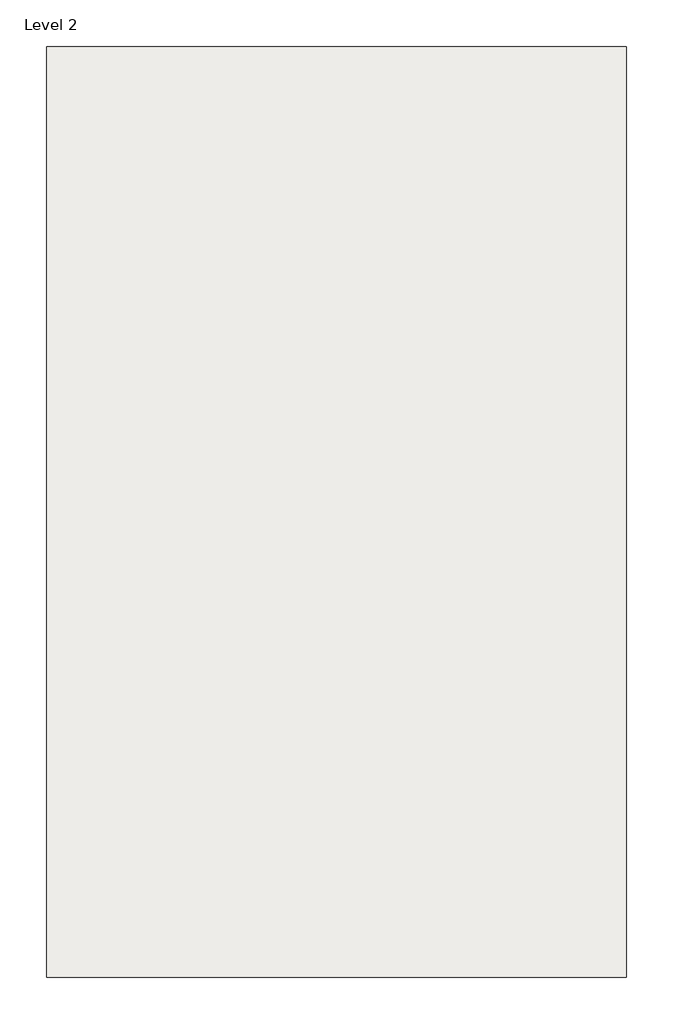
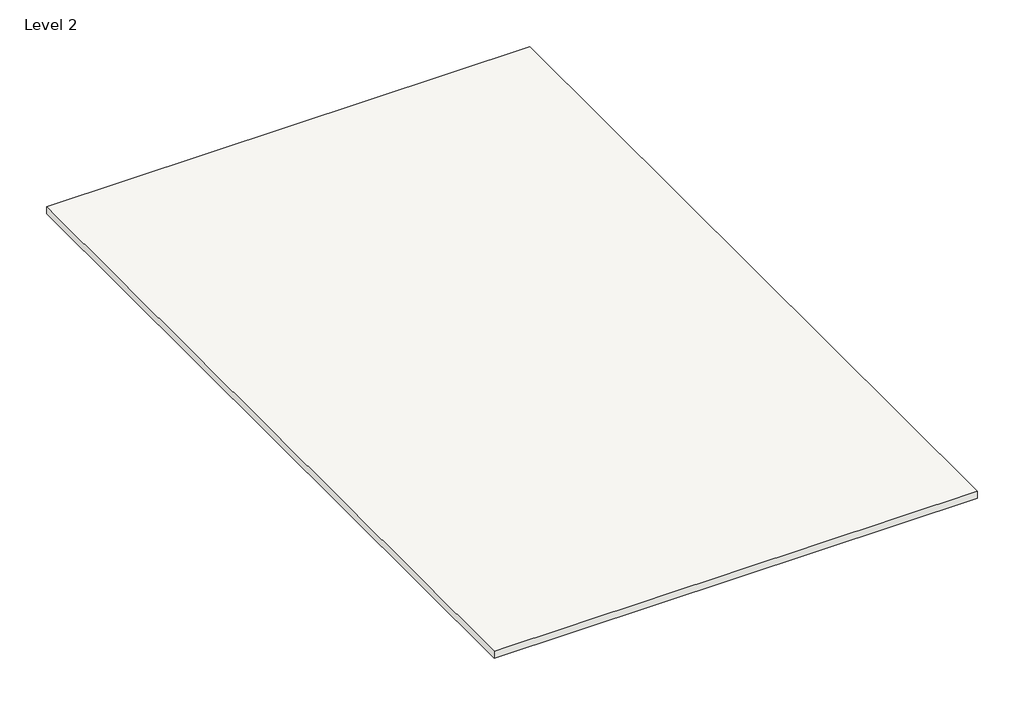
# One storey, incomplete: 1 roof.
"""IFC4 building model written with IfcOpenShell, lengths in millimetres."""

from ifc_helpers import new_model, si_unit, frame, origin, place, context, project, spatial, polyline, outline, extrude, element, save

model = new_model("IFC4")

# Units and contexts
model_context = context("Model", 3, world=origin())
ifc_project = project(units=[si_unit("LENGTHUNIT", "METRE", prefix="MILLI")], contexts=[model_context])

# Site, building, storey
site = spatial("IfcSite", under=ifc_project)
building = spatial("IfcBuilding", under=site)
storey = spatial("IfcBuildingStorey", under=building, Name="Level 2", Elevation=3048.0)

# Roof
placement = place(None, origin())
element("IfcRoof", 1, ObjectType="ROOF 6\"", at=placement, inside=storey, context=model_context, shape_type="SweptSolid", body=[
    extrude(outline(polyline([(-6128.0415352, 7411.3230313), (3625.5584648, 7411.3230313), (3625.5584648, -8235.0769687), (-6128.0415352, -8235.0769687), (-6128.0415352, 7411.3230313)])), frame((0.0, 0.0, 3048.0), z_axis=(0.0, 0.0, 1.0), x_axis=(1.0, 0.0, 0.0)), (0.0, 0.0, 1.0), 152.4),
])

save(model, "model.ifc")

# Revit data of these elements
# Type "ROOF 6\""
#   Assembly Code = "B1020"
#   Layers, outside or top first: 0' - 6" no material (function 1)
# Element 1 (IfcRoof, "ROOF 6\"")
#   built-in parameter 1001705 = 10.5 (stored number, unit not read)
#   built-in parameter 1001710 = 33615
#   Phase Created = New Construction
#   Materials on its faces: "Default Roof", "Door - Panel"
# Materials
#   "Default Roof": colour RGB 88 101 114, transparency 0, Cost = 0
#   "Door - Panel": class "Wood", colour RGB 210 159 95, transparency 0, Cost = 0
